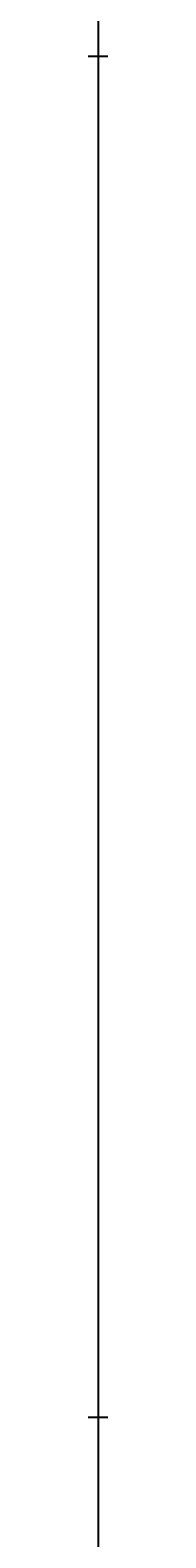
# Model space of a CAD drawing. Units: inches. Extents: x 35362 to 73946, y 43607 to 67532.
# Tile 27 of 134: x 48373 to 48373, y 46091 to 46564. Entities that reach past the tile are written whole.
import ezdxf

# ---------------------------------------------------------------- set-up
doc = ezdxf.new("R2010")
doc.units = ezdxf.units.IN
doc.header["$MEASUREMENT"] = 0
doc.layers.add('A-ANNO-DIMS', color=2, linetype='Continuous', lineweight=18)
doc.styles.get("Standard").update_dxf_attribs({"font": 'arial.ttf'})
doc.dimstyles.get("Standard").update_dxf_attribs({"dimtxt": 0.18, "dimasz": 0.18, "dimexe": 0.18, "dimexo": 0.0625, "dimgap": 0.09, "dimtad": 0, "dimtih": 1, "dimtoh": 1, "dimdec": 4, "dimzin": 0, "dimdsep": 46, "dimtxsty": 'Standard', "dimcen": 0.09, "dimadec": 0, "dimazin": 0, "dimtfac": 1, "dimtdec": 4, "dimtofl": 0, "dimtmove": 0, "dimatfit": 3, "dimfxl": 1, "dimtolj": 1, "dimtzin": 0, "dimarcsym": 0})

# ---------------------------------------------------------------- blocks, each defined once
blk = doc.blocks.new('*D5')
at = {"layer": 'A-ANNO-DIMS', "color": 0, "lineweight": -2, "transparency": 16777216}
for p, q in [((37121.95, 46919.32), (37121.95, 43606.68)), ((69871.5, 45449.83), (69871.5, 43606.68)), ((37122.13, 43606.86), (53496.29, 43606.86)), ((69871.32, 43606.86), (53497.15, 43606.86))]:
    blk.add_line(p, q, dxfattribs=at)
at = {"layer": 'A-ANNO-DIMS', "color": 0, "transparency": 16777216}
for points in [[(37122.13, 43606.89), (37122.13, 43606.83), (37121.95, 43606.86)], [(69871.32, 43606.89), (69871.32, 43606.83), (69871.5, 43606.86)]]:
    blk.add_solid(points, dxfattribs=at)
at = {"layer": 'Defpoints', "color": 0, "transparency": 16777216}
for p in [(37121.95, 46919.38), (69871.5, 45449.89), (69871.5, 43606.86)]:
    blk.add_point(p, dxfattribs=at)
at = {"layer": 'A-ANNO-DIMS', "color": 0, "transparency": 16777216, "insert": (53496.72, 43606.86), "char_height": 0.18, "attachment_point": 5}
blk.add_mtext('\\A1;32750', dxfattribs=at)
blk = doc.blocks.new('*D11')
at = {"layer": 'A-ANNO-DIMS', "color": 0, "lineweight": -2, "transparency": 16777216}
for p, q in [((47978.66, 56028.77), (47978.66, 43606.68)), ((53109.76, 56028.77), (53109.76, 43606.68)), ((47978.84, 43606.86), (50543.87, 43606.86)), ((53109.58, 43606.86), (50544.55, 43606.86))]:
    blk.add_line(p, q, dxfattribs=at)
at = {"layer": 'A-ANNO-DIMS', "color": 0, "transparency": 16777216}
for points in [[(47978.84, 43606.89), (47978.84, 43606.83), (47978.66, 43606.86)], [(53109.58, 43606.89), (53109.58, 43606.83), (53109.76, 43606.86)]]:
    blk.add_solid(points, dxfattribs=at)
at = {"layer": 'Defpoints', "color": 0, "transparency": 16777216}
for p in [(47978.66, 56028.84), (53109.76, 56028.84), (53109.76, 43606.86)]:
    blk.add_point(p, dxfattribs=at)
at = {"layer": 'A-ANNO-DIMS', "color": 0, "transparency": 16777216, "insert": (50544.21, 43606.86), "char_height": 0.18, "attachment_point": 5}
blk.add_mtext('\\A1;5131', dxfattribs=at)
blk = doc.blocks.new('*D27')
at = {"layer": 'A-ANNO-DIMS', "color": 0, "lineweight": -2, "transparency": 16777216}
for p, q in [((47978.66, 56028.77), (47978.66, 43606.68)), ((48373.49, 53428.96), (48373.49, 43606.68)), ((47978.84, 43606.86), (48175.68, 43606.86)), ((48373.31, 43606.86), (48176.47, 43606.86))]:
    blk.add_line(p, q, dxfattribs=at)
at = {"layer": 'A-ANNO-DIMS', "color": 0, "transparency": 16777216}
for points in [[(47978.84, 43606.89), (47978.84, 43606.83), (47978.66, 43606.86)], [(48373.31, 43606.89), (48373.31, 43606.83), (48373.49, 43606.86)]]:
    blk.add_solid(points, dxfattribs=at)
at = {"layer": 'Defpoints', "color": 0, "transparency": 16777216}
for p in [(47978.66, 56028.84), (48373.49, 53429.02), (48373.49, 43606.86)]:
    blk.add_point(p, dxfattribs=at)
at = {"layer": 'A-ANNO-DIMS', "color": 0, "transparency": 16777216, "insert": (48176.08, 43606.86), "char_height": 0.18, "attachment_point": 5}
blk.add_mtext('\\A1;394.8', dxfattribs=at)
blk = doc.blocks.new('*D67')
at = {"layer": 'A-ANNO-DIMS', "color": 0, "lineweight": -2, "transparency": 16777216}
for p, q in [((56873.54, 53351.53), (35361.77, 53351.53)), ((35361.95, 53351.35), (35361.95, 49400.89)), ((35361.95, 45450.07), (35361.95, 49400.53)), ((53793.58, 45449.89), (35361.77, 45449.89))]:
    blk.add_line(p, q, dxfattribs=at)
at = {"layer": 'A-ANNO-DIMS', "color": 0, "transparency": 16777216}
for points in [[(35361.92, 53351.35), (35361.98, 53351.35), (35361.95, 53351.53)], [(35361.92, 45450.07), (35361.98, 45450.07), (35361.95, 45449.89)]]:
    blk.add_solid(points, dxfattribs=at)
at = {"layer": 'Defpoints', "color": 0, "transparency": 16777216}
for p in [(35361.95, 53351.53), (56873.6, 53351.53), (53793.64, 45449.89)]:
    blk.add_point(p, dxfattribs=at)
at = {"layer": 'A-ANNO-DIMS', "color": 0, "transparency": 16777216, "insert": (35361.95, 49400.71), "char_height": 0.18, "attachment_point": 5}
blk.add_mtext('\\A1;7901.6', dxfattribs=at)
blk = doc.blocks.new('*D76')
at = {"layer": 'A-ANNO-DIMS', "color": 0, "lineweight": -2, "transparency": 16777216}
for p, q in [((54052.84, 46555.29), (35361.77, 46555.29)), ((35361.95, 46555.11), (35361.95, 46342.27)), ((35361.95, 46129.06), (35361.95, 46341.9)), ((53793.58, 46128.88), (35361.77, 46128.88))]:
    blk.add_line(p, q, dxfattribs=at)
at = {"layer": 'A-ANNO-DIMS', "color": 0, "transparency": 16777216}
for points in [[(35361.92, 46555.11), (35361.98, 46555.11), (35361.95, 46555.29)], [(35361.92, 46129.06), (35361.98, 46129.06), (35361.95, 46128.88)]]:
    blk.add_solid(points, dxfattribs=at)
at = {"layer": 'Defpoints', "color": 0, "transparency": 16777216}
for p in [(35361.95, 46555.29), (54052.9, 46555.29), (53793.64, 46128.88)]:
    blk.add_point(p, dxfattribs=at)
at = {"layer": 'A-ANNO-DIMS', "color": 0, "transparency": 16777216, "insert": (35361.95, 46342.09), "char_height": 0.18, "attachment_point": 5}
blk.add_mtext('\\A1;426.4', dxfattribs=at)
blk = doc.blocks.new('*D90')
at = {"layer": 'A-ANNO-DIMS', "color": 0, "lineweight": -2, "transparency": 16777216}
for p, q in [((53707.72, 47291.29), (35361.77, 47291.29)), ((35361.95, 47291.11), (35361.95, 46710.26)), ((35361.95, 46129.06), (35361.95, 46709.9)), ((53793.58, 46128.88), (35361.77, 46128.88))]:
    blk.add_line(p, q, dxfattribs=at)
at = {"layer": 'A-ANNO-DIMS', "color": 0, "transparency": 16777216}
for points in [[(35361.92, 47291.11), (35361.98, 47291.11), (35361.95, 47291.29)], [(35361.92, 46129.06), (35361.98, 46129.06), (35361.95, 46128.88)]]:
    blk.add_solid(points, dxfattribs=at)
at = {"layer": 'Defpoints', "color": 0, "transparency": 16777216}
for p in [(53707.78, 47291.29), (35361.95, 46128.88), (53793.64, 46128.88)]:
    blk.add_point(p, dxfattribs=at)
at = {"layer": 'A-ANNO-DIMS', "color": 0, "transparency": 16777216, "insert": (35361.95, 46710.08), "char_height": 0.18, "attachment_point": 5}
blk.add_mtext('\\A1;1162.4', dxfattribs=at)

msp = doc.modelspace()

# ---------------------------------------------------------------- dimensions: what is measured, and where the dimension line sits
at = {"layer": 'A-ANNO-DIMS'}
for base, p1, p2, override, picture, middle in [((53109.76, 43606.859), (47978.665, 56028.836), (53109.76, 56028.836), {"dimdec": 0, "dimlfac": 1, "dimrnd": 0, "dimzin": 0, "dimdsep": 46, "dimlunit": 2}, '*D11', (50544.212, 43606.859)), ((48373.492, 43606.859), (47978.665, 56028.836), (48373.492, 53429.019), {"dimdec": 1, "dimlfac": 1, "dimrnd": 0, "dimzin": 0, "dimdsep": 46, "dimlunit": 2}, '*D27', (48176.078, 43606.859)), ((69871.496, 43606.859), (37121.949, 46919.381), (69871.496, 45449.894), {"dimdec": 0, "dimlfac": 1, "dimrnd": 0, "dimzin": 0, "dimdsep": 46, "dimlunit": 2}, '*D5', (53496.723, 43606.859))]:
    dim = msp.add_linear_dim(base=base, p1=p1, p2=p2, dimstyle='Standard', override=override, dxfattribs=at)
    dim.commit()
    dim.dimension.update_dxf_attribs({"geometry": picture, "text_midpoint": middle})
for base, p1, p2, picture, middle in [((35361.949, 53351.529), (53793.638, 45449.894), (56873.602, 53351.529), '*D67', (35361.949, 49400.712)), ((35361.949, 46128.878), (53707.781, 47291.285), (53793.638, 46128.878), '*D90', (35361.949, 46710.081)), ((35361.949, 46555.293), (53793.638, 46128.878), (54052.899, 46555.293), '*D76', (35361.949, 46342.086))]:
    dim = msp.add_linear_dim(base=base, p1=p1, p2=p2, angle=90, dimstyle='Standard', override={"dimdec": 1, "dimlfac": 1, "dimrnd": 0, "dimzin": 0, "dimdsep": 46, "dimlunit": 2}, dxfattribs=at)
    dim.commit()
    dim.dimension.update_dxf_attribs({"geometry": picture, "text_midpoint": middle})

doc.saveas('drawing.dxf')
